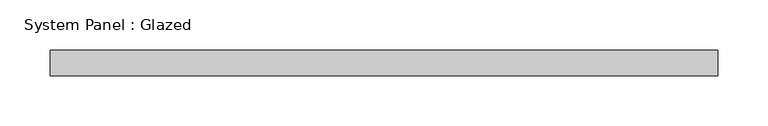
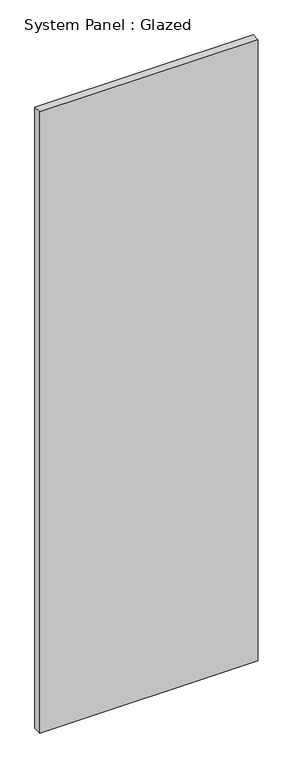
"""IFC4 building model written with IfcOpenShell, lengths in millimetres: plate geometry, System Panel : Glazed."""

from ifc_helpers import new_model, si_unit, origin, origin_with_axes, place, context, project, spatial, polyline, outline, extrude, source, transform, mapped, element, save


def system_panel_glazed_a68fd5c2(model_context):
    return source(origin(), model_context, "Body", "SweptSolid", [
        extrude(outline(polyline([(333.375, 19.05), (-333.375, 19.05), (-333.375, 44.45), (333.375, 44.45), (333.375, 19.05)])), origin_with_axes(), (0.0, 0.0, 1.0), 2006.6),
    ])


if __name__ == "__main__":
    model = new_model("IFC4")
    model_context = context("Model", 3, world=origin())
    ifc_project = project(units=[si_unit("LENGTHUNIT", "METRE", prefix="MILLI")], contexts=[model_context])
    site = spatial("IfcSite", under=ifc_project)
    building = spatial("IfcBuilding", under=site)
    placement = place(None, origin())
    system_panel_glazed_shape = system_panel_glazed_a68fd5c2(model_context)
    element("IfcPlate", 1, ObjectType="System Panel : Glazed", at=placement, inside=building, context=model_context, shape_type="MappedRepresentation", body=[
        mapped(system_panel_glazed_shape, transform((0.0, 0.0, 0.0), x_axis=(1.0, 0.0, 0.0), y_axis=(0.0, 1.0, 0.0), z_axis=(0.0, 0.0, 1.0))),
    ])
    save(model, "model.ifc")

# Revit data of these elements
# Type "System Panel : Glazed"
#   Construction Type Id = "GSP4R"
#   Analytic Construction = "1/8 in Pilkington single glazing"
#   Visual Light Transmittance = 0.9
#   Solar Heat Gain Coefficient = 0.86
#   Heat Transfer Coefficient (U) = 1.18115 BTU/(h·ft²·°F)
#   Define Thermal Properties by = 1
# Element 1 (IfcPlate, "System Panel : Glazed")
#   Materials on its faces: "Glass"
# Materials
#   "Glass": class "Glass", colour RGB 0 128 192, transparency 0.75, Description = "Soda Lime Glass", Cost = 0
